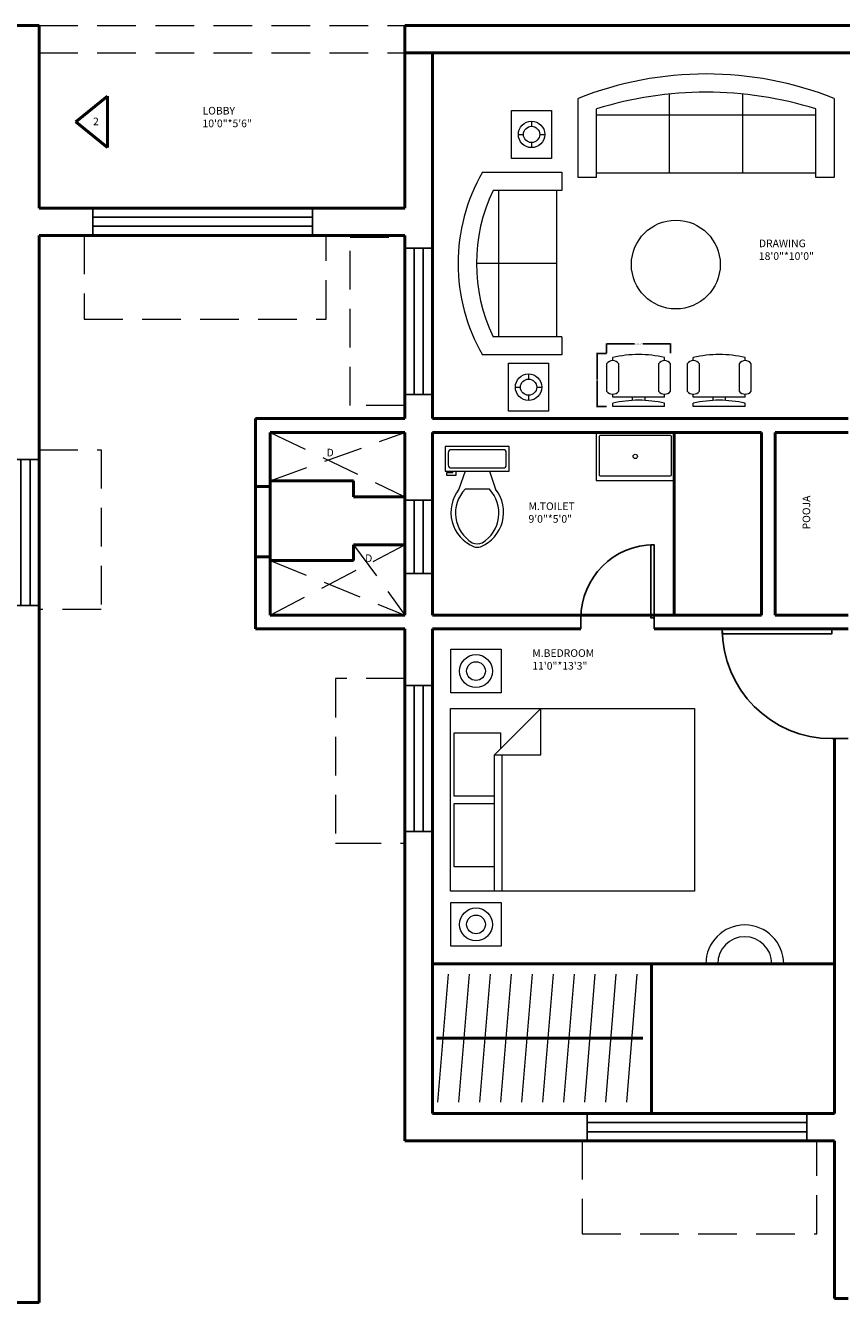
# Model space of a CAD drawing. Units: inches. Extents: x 291 to 2631, y 456 to 2623.
# Tile 4 of 22: x 900 to 1167, y 512 to 931. Entities that reach past the tile are written whole.
import ezdxf

# ---------------------------------------------------------------- set-up
doc = ezdxf.new("R2010")
doc.units = ezdxf.units.IN
doc.linetypes.add('DASHED', pattern=[19.05, 12.7, -6.35])
for name, color, linetype, lineweight in [('A-ANNO-DIMS', 2, 'Continuous', 18), ('A-ANNO-TEXT', 3, 'Continuous', 25), ('A-AREA-IDEN', 7, 'Continuous', 25), ('A-DOOR', 3, 'Continuous', 25), ('A-FLOR-FIXT', 9, 'Continuous', 18), ('A-FLOR-OVHD', 1, 'DASHED', 18), ('A-FURN', 8, 'Continuous', 18), ('A-GLAZ', 4, 'Continuous', 25), ('A-WALL', 7, 'Continuous', 50)]:
    doc.layers.add(name, color=color, linetype=linetype, lineweight=lineweight)
doc.styles.get("Standard").update_dxf_attribs({"font": 'arial.ttf'})
doc.dimstyles.get("Standard").update_dxf_attribs({"dimtxt": 0.18, "dimasz": 0.18, "dimexe": 0.18, "dimexo": 0.0625, "dimgap": 0.09, "dimtad": 0, "dimtih": 1, "dimtoh": 1, "dimdec": 4, "dimzin": 0, "dimdsep": 46, "dimtxsty": 'Standard', "dimcen": 0.09, "dimadec": 0, "dimazin": 0, "dimtfac": 1, "dimtdec": 4, "dimtofl": 0, "dimtmove": 0, "dimatfit": 3, "dimfxl": 1, "dimtolj": 1, "dimtzin": 0, "dimarcsym": 0})

# ---------------------------------------------------------------- blocks, each defined once
blk = doc.blocks.new('*U2')
for p, q in [((0, 0), (0, -6)), ((40, 0), (40, -6))]:
    blk.add_line(p, q)
blk.add_lwpolyline([(0, 0), (0, 40), (1.75, 40), (1.75, 0)], close=True)
blk.add_arc((0, 0), 40, 0, 90)
blk = doc.blocks.new('Sofa - Roundback 7 ft.')
for p, q in [((-12.00002, -32.4421), (-12.00003, -6.5971)), ((11.99997, -32.4421), (11.99998, -6.5971)), ((-36.000027, -34), (-36.000027, -11.4696)), ((35.99998, -34), (35.99998, -11.4696)), ((-35.999844, -13.3819), (35.9998, -13.3819)), ((-36.000027, -32.4421), (35.99998, -32.4421))]:
    blk.add_line(p, q)
for points in [[(-36.000027, -34), (-42.000027, -34), (-42.000027, -8)], [(41.99998, -8), (41.99998, -34), (35.99998, -34)]]:
    blk.add_lwpolyline(points)
for centre, radius, start, end in [((0, -114.25), 114.25, 68.43141, 111.5686), ((-0.00001, -127.1968), 121.1968, 72.72033, 107.2797)]:
    blk.add_arc(centre, radius, start, end)
blk = doc.blocks.new('Sofa - Roundback Loveseat 5 ft.')
for p, q in [((0, -32.44198), (0, -5.99998)), ((-24, -33.99998), (-24, -11.46958)), ((24.00004, -33.99998), (24.00004, -11.46958)), ((-23.9998, -13.38178), (23.99986, -13.38178)), ((-24, -32.44198), (24.00004, -32.44198))]:
    blk.add_line(p, q)
for points in [[(-24, -33.99998), (-30, -33.99998), (-30, -7.99998)], [(30.00004, -7.99998), (30.00004, -33.99998), (24.00004, -33.99998)]]:
    blk.add_lwpolyline(points)
for centre, radius, start, end in [((0, -60.24998), 60.24998, 60.13715, 119.8628), ((0, -61.38438), 55.38444, 64.32083, 115.6792)]:
    blk.add_arc(centre, radius, start, end)
blk = doc.blocks.new('Chair - Desk')
for p, q in [((-8.5, 0), (-8.5, -1)), ((-8.5, 0), (8.5, 0)), ((8.5, 0), (8.5, -1)), ((-8.5, -3), (-8.5, -4)), ((-8.5, -3), (8.5, -3)), ((-2, -3), (-2, -1.9355)), ((2, -1.9576), (2, -3)), ((8.5, -3), (8.5, -4)), ((-10.5, -5), (-10.5, -14)), ((-6.5, -14), (-6.5, -5)), ((6.5, -5), (6.5, -14)), ((10.5, -14), (10.5, -5)), ((-8.5, -15), (-8.5, -16)), ((8.5, -15), (8.5, -16))]:
    blk.add_line(p, q)
for centre, radius, start, end in [((-8.5, -6.5), 2.5, 36.8699, 143.1301), ((0, 34.625), 36.625, 256.5803, 283.4197), ((8.5, -6.5), 2.5, 36.8699, 143.1301), ((-8.5, -12.5), 2.5, 216.8699, 323.1301), ((0, 19.625), 36.625, 256.5803, 283.4197), ((8.5, -12.5), 2.5, 216.8699, 323.1301)]:
    blk.add_arc(centre, radius, start, end)
blk = doc.blocks.new('Toilet - top')
for p, q in [((9.5, -6), (9.5, -2)), ((-8, -8.5), (-8, -8)), ((-7, -8), (-7, -9.5)), ((-4, -8), (-6, -14)), ((4, -8), (6, -14)), ((-10, -8.5), (-8, -8.5)), ((-10, -9.5), (-10, -8.5)), ((-7, -9.5), (-10, -9.5)), ((4, -14), (-4, -14))]:
    blk.add_line(p, q)
blk.add_lwpolyline([(10.5, -8), (10.5, 0), (-10.5, 0), (-10.5, -8)], close=True)
for points in [[(-9.5, -2), (-9.5, -6)], [(8.5, -1), (-8.5, -1)], [(-8.5, -7), (8.5, -7)]]:
    blk.add_lwpolyline(points)
for centre, radius, start, end in [((-8.62, -1.88), 0.884, 81.8699, 188.1301), ((8.62, -1.88), 0.884, 351.8699, 98.1301), ((-8.62, -6.12), 0.884, 171.8699, 278.1301), ((8.62, -6.12), 0.884, 261.8699, 8.1301), ((3.52, -21.58), 12.17, 141.4691, 247.9714), ((4.2, -21.82), 11.33, 136.3677, 238.9468), ((-3.52, -21.58), 12.17, 292.0284, 38.5307), ((-4.2, -21.82), 11.33, 301.053, 43.6321), ((0, -27.88), 4, 245.7318, 294.2682), ((0, -29), 4, 254.8605, 285.1395)]:
    blk.add_arc(centre, radius, start, end)
blk = doc.blocks.new('Bed - Queen')
for p, q in [((0, -80.00003), (0, 0)), ((0, 0), (59.99999, 0)), ((59.99999, 0), (59.99999, -80.00003)), ((7.99999, -1.2), (28.79998, -1.2)), ((7.99999, -14.4), (7.99999, -1.2)), ((28.79998, -1.2), (28.79998, -14.4)), ((31.19999, -1.2), (51.99999, -1.2)), ((31.19999, -14.4), (31.19999, -1.2)), ((51.99999, -1.2), (51.99999, -16.4)), ((0, -14.4), (44.8, -14.4)), ((59.99999, -29.6), (44.8, -14.4)), ((44.8, -14.4), (44.8, -29.6)), ((51.99999, -16.4), (46.79936, -16.4)), ((44.8, -16.8), (0, -16.8)), ((44.8, -29.6), (59.99999, -29.6)), ((59.99999, -80.00003), (0, -80.00003))]:
    blk.add_line(p, q)
blk = doc.blocks.new('WIN-1800')
for p, q in [((0, 9), (72, 9)), ((0, 0), (0, 9)), ((72, 9), (72, 0)), ((0, 6), (72, 6)), ((72, 3), (0, 3)), ((72, 0), (0, 0))]:
    blk.add_line(p, q)
blk = doc.blocks.new('WIN-1200')
for p, q in [((0, 0), (0, 48)), ((0, 48), (9, 48)), ((3, 0), (3, 48)), ((6, 48), (6, 0)), ((9, 48), (9, 0)), ((9, 0), (0, 0))]:
    blk.add_line(p, q)
blk = doc.blocks.new('WIN-600')
for p, q in [((24, 9), (0, 9)), ((0, 9), (0, 0)), ((24, 0), (24, 9)), ((24, 6), (0, 6)), ((0, 3), (24, 3)), ((0, 0), (24, 0))]:
    blk.add_line(p, q)
blk = doc.blocks.new('LAMP-A')
for p, q in [((6.55, 12.25), (6.55, 10.56)), ((2.2, 7.9), (3.88, 7.9)), ((6.55, 5.24), (6.55, 3.56)), ((9.21, 7.9), (10.89, 7.9))]:
    blk.add_line(p, q)
blk.add_lwpolyline([(0, 15.8), (13.09, 15.8), (13.09, 0), (0, 0)], close=True)
for radius in [4.34, 2.66]:
    blk.add_circle((6.55, 7.9), radius)
blk = doc.blocks.new('*D40')
at = {"layer": 'A-ANNO-DIMS', "color": 0, "lineweight": -2, "transparency": 16777216}
for p, q in [((1090.2, 823.42), (1090.2, 826.68)), ((1090.38, 826.5), (1099.37, 826.5)), ((1111.02, 826.5), (1102.03, 826.5)), ((1111.2, 823.42), (1111.2, 826.68))]:
    blk.add_line(p, q, dxfattribs=at)
at = {"layer": 'A-ANNO-DIMS', "color": 0, "transparency": 16777216}
for points in [[(1090.38, 826.53), (1090.38, 826.47), (1090.2, 826.5)], [(1111.02, 826.53), (1111.02, 826.47), (1111.2, 826.5)]]:
    blk.add_solid(points, dxfattribs=at)
at = {"layer": 'DEFPOINTS', "color": 0, "transparency": 16777216}
for p in [(1090.2, 826.5), (1090.2, 823.35), (1111.2, 823.35)]:
    blk.add_point(p, dxfattribs=at)
at = {"layer": 'A-ANNO-DIMS', "color": 0, "transparency": 16777216, "insert": (1100.7, 826.5), "char_height": 0.18, "attachment_point": 5}
blk.add_mtext('\\A1;DESK CHAIR 21 TYP.', dxfattribs=at)
blk = doc.blocks.new('*D41')
at = {"layer": 'A-ANNO-DIMS', "color": 0, "lineweight": -2, "transparency": 16777216}
for p, q in [((1090.14, 823.35), (1086.87, 823.35)), ((1087.05, 823.17), (1087.05, 814.87)), ((1087.05, 806.2), (1087.05, 814.51)), ((1090.14, 806.02), (1086.87, 806.02))]:
    blk.add_line(p, q, dxfattribs=at)
at = {"layer": 'A-ANNO-DIMS', "color": 0, "transparency": 16777216}
for points in [[(1087.02, 823.17), (1087.08, 823.17), (1087.05, 823.35)], [(1087.02, 806.2), (1087.08, 806.2), (1087.05, 806.02)]]:
    blk.add_solid(points, dxfattribs=at)
at = {"layer": 'DEFPOINTS', "color": 0, "transparency": 16777216}
for p in [(1090.2, 823.35), (1087.05, 806.02), (1090.2, 806.02)]:
    blk.add_point(p, dxfattribs=at)
at = {"layer": 'A-ANNO-DIMS', "color": 0, "transparency": 16777216, "insert": (1087.05, 814.69), "char_height": 0.18, "attachment_point": 5}
blk.add_mtext('\\A1;17 TYP.', dxfattribs=at)

msp = doc.modelspace()

# ---------------------------------------------------------------- linework, layer by layer
at = {"layer": 'A-FLOR-OVHD'}
for p, q in [((904, 930.98), (1024, 930.98)), ((904, 921.98), (1024, 921.98)), ((918.71, 862.1), (918.71, 834.68)), ((998.19, 834.68), (998.19, 862.1)), ((1006.04, 806.27), (1006.04, 861.55)), ((1006.04, 861.55), (1024, 861.55)), ((918.71, 834.68), (998.19, 834.68)), ((1024, 806.27), (1006.04, 806.27)), ((979.83, 797.48), (1024, 776.35)), ((979.83, 781.62), (1024, 797.48)), ((904, 791.76), (924.28, 791.76)), ((924.28, 791.76), (924.28, 739.31)), ((979.83, 737.48), (1024, 760.62)), ((1007.15, 760.62), (1024, 737.48)), ((979.83, 755.46), (1024, 737.48)), ((924.28, 739.31), (904, 739.31)), ((1024, 716.67), (1001.18, 716.67)), ((1001.18, 716.67), (1001.18, 662.73)), ((1001.18, 662.73), (1003.47, 662.73)), ((1003.47, 662.73), (1024, 662.73)), ((1024, 662.73), (1024, 662.73)), ((1082.11, 564.98), (1082.11, 534.48)), ((1159.22, 534.48), (1159.22, 564.98)), ((1082.11, 534.48), (1159.22, 534.48))]:
    msp.add_line(p, q, dxfattribs=at)
at = {"layer": 'A-FURN'}
for p, q in [((1034.82, 577.75), (1038.28, 619.73)), ((1041.71, 577.75), (1045.17, 619.73)), ((1048.6, 577.75), (1052.05, 619.73)), ((1055.48, 577.75), (1058.94, 619.73)), ((1062.37, 577.75), (1065.82, 619.73)), ((1069.26, 577.75), (1072.71, 619.73)), ((1076.14, 577.75), (1079.6, 619.73)), ((1083.03, 577.75), (1086.48, 619.73)), ((1089.91, 577.75), (1093.37, 619.73)), ((1096.8, 577.75), (1100.26, 619.73))]:
    msp.add_line(p, q, dxfattribs=at)
for points in [[(1112.37, 797.48), (1086.79, 797.48), (1086.79, 781.7), (1112.37, 781.7)], [(1039.08, 726.3), (1055.56, 726.3), (1055.56, 712.01), (1039.08, 712.01)], [(1039.09, 643.18), (1055.57, 643.18), (1055.57, 628.88), (1039.09, 628.88)]]:
    msp.add_lwpolyline(points, close=True, dxfattribs=at)
msp.add_lwpolyline([(1088.3, 796.58), (1110.9, 796.58, -0.414214), (1111.4, 796.08), (1111.4, 783.57, -0.414214), (1110.9, 783.07), (1088.3, 783.07, -0.414214), (1087.8, 783.57), (1087.8, 796.08, -0.414214)], format="xyb", close=True, dxfattribs=at)
for centre, radius in [((1112.9, 852.56), 14.57), ((1099.58, 789.59), 0.728), ((1047.32, 719.16), 5.39), ((1047.32, 719.16), 3.08), ((1047.33, 636.03), 5.39), ((1047.33, 636.03), 3.08)]:
    msp.add_circle(centre, radius, dxfattribs=at)
for radius in [12.77, 8.89]:
    msp.add_arc((1135.52, 623.08), radius, 0, 180, dxfattribs=at)
at = {"layer": 'A-WALL'}
for p, q in [((904, 930.98), (616.5, 930.98)), ((904, 871.1), (904, 930.98)), ((1989.87, 930.98), (1024, 930.98)), ((1024, 930.98), (1024, 871.1)), ((1033, 921.98), (1024, 921.98)), ((1033, 921.98), (1033, 801.98)), ((1409.5, 921.98), (1033, 921.98)), ((915.99, 899.36), (926.45, 907.81)), ((926.45, 907.81), (926.45, 890.92)), ((926.45, 890.92), (915.99, 899.36)), ((1024, 871.1), (904, 871.1)), ((1024, 862.1), (904, 862.1)), ((904, 862.1), (904, 511.98)), ((1024, 862.1), (1024, 801.98)), ((1024, 801.98), (974.96, 801.98)), ((974.96, 801.98), (974.96, 732.98)), ((1169.5, 801.98), (1033, 801.98)), ((1024, 797.48), (979.83, 797.48)), ((979.83, 797.48), (979.83, 737.48)), ((1024, 797.48), (1024, 737.48)), ((1033, 797.48), (1033, 737.48)), ((1141, 797.48), (1033, 797.48)), ((1112.37, 797.48), (1112.37, 737.48)), ((1141, 797.48), (1141, 737.48)), ((1145.5, 797.48), (1145.5, 737.48)), ((1169.5, 797.48), (1145.5, 797.48)), ((979.83, 779.67), (974.96, 779.67)), ((979.83, 781.62), (1007.15, 781.62)), ((1007.15, 781.62), (1007.15, 776.35)), ((1007.15, 776.35), (1024, 776.35)), ((1007.15, 755.46), (1007.15, 760.62)), ((1007.15, 760.62), (1024, 760.62)), ((979.83, 756.59), (974.96, 756.59)), ((979.83, 755.46), (1007.15, 755.46)), ((979.83, 737.48), (1024, 737.48)), ((1141, 737.48), (1033, 737.48)), ((1169.5, 737.48), (1145.5, 737.48)), ((974.96, 732.98), (1024, 732.98)), ((1024, 732.98), (1024, 564.98)), ((1033, 732.98), (1033, 573.98)), ((1081.76, 732.98), (1033, 732.98)), ((1169.5, 732.98), (1105.76, 732.98)), ((1165, 696.98), (1165, 573.98)), ((1033, 623.08), (1165, 623.08)), ((1104.95, 623.08), (1104.95, 573.98)), ((1034.39, 598.74), (1102.12, 598.74)), ((1165, 573.98), (1033, 573.98)), ((1165, 564.98), (1024, 564.98)), ((1165, 564.98), (1165, 513.24)), ((904, 511.98), (753, 511.98)), ((1165, 513.24), (1169.5, 513.24))]:
    msp.add_line(p, q, dxfattribs=at)

# ---------------------------------------------------------------- block references
at = {"layer": 'A-DOOR', "xscale": -0.6, "yscale": 0.6, "zscale": 0.6}
msp.add_blockref('*U2', (1105.76, 736.58), dxfattribs=at)
at = {"layer": 'A-DOOR', "xscale": -0.9, "yscale": 0.9, "zscale": 0.9, "rotation": 90}
msp.add_blockref('*U2', (1164.1, 732.98), dxfattribs=at)
at = {"layer": 'A-FLOR-FIXT'}
msp.add_blockref('Toilet - top', (1047.73, 792.8), dxfattribs=at)
at = {"layer": 'A-FURN'}
for name, p in [('Sofa - Roundback 7 ft.', (1122.85, 915.08)), ('LAMP-A', (1059.02, 887.35)), ('LAMP-A', (1058.03, 804.41))]:
    msp.add_blockref(name, p, dxfattribs=at)
for name, p, rotation in [('Sofa - Roundback Loveseat 5 ft.', (1041.46, 852.88), 90), ('Chair - Desk', (1100.7, 806.02), 180), ('Chair - Desk', (1127.14, 806.02), 180), ('Bed - Queen', (1038.99, 646.92), 90)]:
    msp.add_blockref(name, p, dxfattribs=dict(at, rotation=rotation))
at = {"layer": 'A-GLAZ'}
for name, p in [('WIN-1800', (921.64, 862.1)), ('WIN-1200', (1024, 809.87)), ('WIN-1200', (895, 740.63)), ('WIN-1200', (1024, 666.47)), ('WIN-1800', (1083.84, 564.98))]:
    msp.add_blockref(name, p, dxfattribs=at)
at = {"layer": 'A-GLAZ', "rotation": 269.9999999999978}
msp.add_blockref('WIN-600', (1024, 775.19), dxfattribs=at)

# ---------------------------------------------------------------- texts
at = {"layer": 'A-ANNO-TEXT', "char_height": 2.5, "attachment_point": 1}
for s, width, insert in [('2', 4.7631, (921.66, 900.76)), ('D', 5.1515, (998.29, 792.11)), ('D', 2.456, (1010.94, 757.43))]:
    msp.add_mtext_dynamic_manual_height_columns(s, width=width, gutter_width=12.5, heights=[0], dxfattribs=dict(at, insert=insert))
at = {"layer": 'A-AREA-IDEN', "char_height": 2.5, "attachment_point": 1}
for s, width, insert in [('LOBBY\\P10\'0"*5\'6"', 64.6747, (957.58, 904.28)), ('DRAWING\\P18\'0"*10\'0"', 61.3955, (1140.15, 860.74)), ('M.TOILET\\P9\'0"*5\'0"', 42.0486, (1064.55, 774.5)), ('M.BEDROOM\\P11\'0"*13\'3"', 49.3325, (1065.8, 726.31))]:
    msp.add_mtext_dynamic_manual_height_columns(s, width=width, gutter_width=12.5, heights=[0], dxfattribs=dict(at, insert=insert))
at = {"layer": 'A-AREA-IDEN', "insert": (1154.5, 765.62), "char_height": 2.5, "attachment_point": 1, "rotation": 90}
msp.add_mtext_dynamic_manual_height_columns('POOJA', width=20.6812, gutter_width=12.5, heights=[0], dxfattribs=at)

# ---------------------------------------------------------------- dimensions: what is measured, and where the dimension line sits
at = {"layer": 'A-ANNO-DIMS'}
for base, p1, p2, angle, text, picture, middle in [((1090.2, 826.5), (1111.2, 823.35), (1090.2, 823.35), 180, 'DESK CHAIR <> TYP.', '*D40', (1100.7, 826.5)), ((1087.05, 806.02), (1090.2, 823.35), (1090.2, 806.02), 270, '<> TYP.', '*D41', (1087.05, 814.69))]:
    dim = msp.add_linear_dim(base=base, p1=p1, p2=p2, angle=angle, text=text, dimstyle='Standard', override={"dimdec": 0, "dimlfac": 1, "dimrnd": 0, "dimzin": 0, "dimdsep": 46, "dimlunit": 2}, dxfattribs=at)
    dim.commit()
    dim.dimension.update_dxf_attribs({"geometry": picture, "text_midpoint": middle})

doc.saveas('drawing.dxf')
